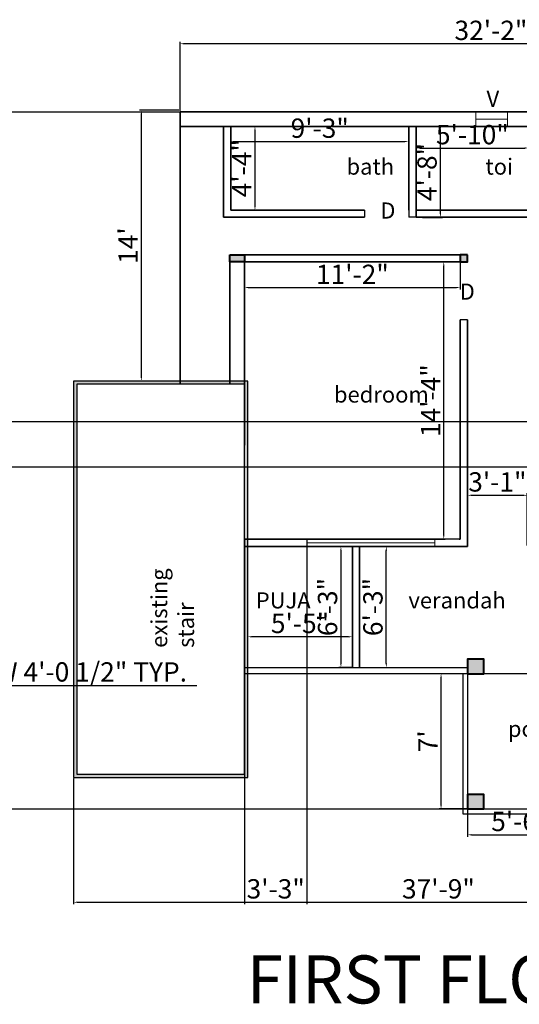
# Model space of a CAD drawing. Units: inches. Extents: x 1989 to 3287, y 1752 to 2384.
# Tile 4 of 5: x 2638 to 2948, y 1752 to 2364. Entities that reach past the tile are written whole.
import ezdxf

# ---------------------------------------------------------------- set-up
doc = ezdxf.new("R2010")
doc.units = ezdxf.units.IN
for name, color, linetype, lineweight in [('A-ANNO-DIMS', 2, 'Continuous', 18), ('A-ANNO-TEXT', 7, 'Continuous', 18), ('A-AREA-IDEN', 7, 'Continuous', 18), ('A-COLS', 1, 'Continuous', 40), ('A-COLS-PATT', 8, 'Continuous', 13), ('A-DOOR', 3, 'Continuous', 25), ('A-FLOR-EDGE', 7, 'Continuous', 25), ('A-FLOR-PATT', 252, 'Continuous', 13), ('A-FLOR-STRS', 7, 'Continuous', 25), ('A-GLAZ', 4, 'Continuous', 18), ('A-WALL', 7, 'Continuous', 35)]:
    doc.layers.add(name, color=color, linetype=linetype, lineweight=lineweight)
doc.styles.get("Standard").update_dxf_attribs({"font": 'arial.ttf'})
doc.dimstyles.new('ISO-25', dxfattribs={"dimtxt": 12, "dimasz": 2.5, "dimexe": 1.25, "dimexo": 0.625, "dimtad": 1, "dimdec": 0, "dimlunit": 4, "dimtxsty": 'Standard', "dimcen": 2.5, "dimadec": 0, "dimazin": 0, "dimtfac": 1, "dimtdec": 0, "dimtmove": 0, "dimatfit": 3, "dimfxl": 1, "dimarcsym": 0})

# ---------------------------------------------------------------- blocks, each defined once
blk = doc.blocks.new('*D18')
at = {"layer": 'A-ANNO-DIMS', "color": 0, "lineweight": -2, "transparency": 16777216}
for p, q in [((2915.08, 1957.68), (2898.02, 1957.68)), ((2899.27, 1876.18), (2899.27, 1955.18)), ((2915.08, 1873.68), (2898.02, 1873.68))]:
    blk.add_line(p, q, dxfattribs=at)
at = {"layer": 'A-ANNO-DIMS', "color": 0, "transparency": 16777216}
for points in [[(2898.85, 1955.18), (2899.68, 1955.18), (2899.27, 1957.68)], [(2898.85, 1876.18), (2899.68, 1876.18), (2899.27, 1873.68)]]:
    blk.add_solid(points, dxfattribs=at)
at = {"layer": 'Defpoints', "color": 0, "transparency": 16777216}
for p in [(2899.27, 1957.68), (2915.71, 1957.68), (2915.71, 1873.68)]:
    blk.add_point(p, dxfattribs=at)
at = {"layer": 'A-ANNO-DIMS', "color": 0, "transparency": 16777216, "insert": (2892.64, 1915.68), "char_height": 12, "attachment_point": 5, "rotation": 90}
blk.add_mtext("7'", dxfattribs=at)
blk = doc.blocks.new('*D19')
at = {"layer": 'A-ANNO-DIMS', "color": 0, "lineweight": -2, "transparency": 16777216}
for p, q in [((2915.71, 1873.05), (2915.71, 1856.37)), ((2981.21, 1873.05), (2981.21, 1856.37)), ((2918.21, 1857.62), (2978.71, 1857.62))]:
    blk.add_line(p, q, dxfattribs=at)
at = {"layer": 'A-ANNO-DIMS', "color": 0, "transparency": 16777216}
for points in [[(2918.21, 1858.04), (2918.21, 1857.2), (2915.71, 1857.62)], [(2978.71, 1858.04), (2978.71, 1857.2), (2981.21, 1857.62)]]:
    blk.add_solid(points, dxfattribs=at)
at = {"layer": 'Defpoints', "color": 0, "transparency": 16777216}
for p in [(2915.71, 1873.68), (2981.21, 1873.68), (2981.21, 1857.62)]:
    blk.add_point(p, dxfattribs=at)
at = {"layer": 'A-ANNO-DIMS', "color": 0, "transparency": 16777216, "insert": (2948.46, 1864.37), "char_height": 12, "attachment_point": 5}
blk.add_mtext('5\'-6"', dxfattribs=at)
blk = doc.blocks.new('*D24')
at = {"layer": 'A-ANNO-DIMS', "color": 0, "lineweight": -2, "transparency": 16777216}
for p, q in [((2910.58, 2213.45), (2899.68, 2213.45)), ((2900.93, 2043.68), (2900.93, 2210.95)), ((2910.58, 2041.18), (2899.68, 2041.18))]:
    blk.add_line(p, q, dxfattribs=at)
at = {"layer": 'A-ANNO-DIMS', "color": 0, "transparency": 16777216}
for points in [[(2900.52, 2210.95), (2901.35, 2210.95), (2900.93, 2213.45)], [(2900.52, 2043.68), (2901.35, 2043.68), (2900.93, 2041.18)]]:
    blk.add_solid(points, dxfattribs=at)
at = {"layer": 'Defpoints', "color": 0, "transparency": 16777216}
for p in [(2900.93, 2213.45), (2911.21, 2213.45), (2911.21, 2041.18)]:
    blk.add_point(p, dxfattribs=at)
at = {"layer": 'A-ANNO-DIMS', "color": 0, "transparency": 16777216, "insert": (2894.28, 2127.31), "char_height": 12, "attachment_point": 5, "rotation": 90}
blk.add_mtext('14\'-4"', dxfattribs=at)
blk = doc.blocks.new('*D25')
at = {"layer": 'A-ANNO-DIMS', "color": 0, "lineweight": -2, "transparency": 16777216}
for p, q in [((2777.21, 2212.82), (2777.21, 2196.3)), ((2911.21, 2212.82), (2911.21, 2196.3)), ((2779.71, 2197.55), (2908.71, 2197.55))]:
    blk.add_line(p, q, dxfattribs=at)
at = {"layer": 'A-ANNO-DIMS', "color": 0, "transparency": 16777216}
for points in [[(2779.71, 2197.97), (2779.71, 2197.13), (2777.21, 2197.55)], [(2908.71, 2197.97), (2908.71, 2197.13), (2911.21, 2197.55)]]:
    blk.add_solid(points, dxfattribs=at)
at = {"layer": 'Defpoints', "color": 0, "transparency": 16777216}
for p in [(2777.21, 2213.45), (2911.21, 2213.45), (2911.21, 2197.55)]:
    blk.add_point(p, dxfattribs=at)
at = {"layer": 'A-ANNO-DIMS', "color": 0, "transparency": 16777216, "insert": (2844.21, 2204.2), "char_height": 12, "attachment_point": 5}
blk.add_mtext('11\'-2"', dxfattribs=at)
blk = doc.blocks.new('*D26')
at = {"layer": 'A-ANNO-DIMS', "color": 0, "lineweight": -2, "transparency": 16777216}
for p, q in [((2736.58, 2307.68), (2711.96, 2307.68)), ((2713.21, 2141.99), (2713.21, 2305.18)), ((2736.58, 2139.49), (2711.96, 2139.49))]:
    blk.add_line(p, q, dxfattribs=at)
at = {"layer": 'A-ANNO-DIMS', "color": 0, "transparency": 16777216}
for points in [[(2712.79, 2305.18), (2713.63, 2305.18), (2713.21, 2307.68)], [(2712.79, 2141.99), (2713.63, 2141.99), (2713.21, 2139.49)]]:
    blk.add_solid(points, dxfattribs=at)
at = {"layer": 'Defpoints', "color": 0, "transparency": 16777216}
for p in [(2713.21, 2307.68), (2737.21, 2307.68), (2737.21, 2139.49)]:
    blk.add_point(p, dxfattribs=at)
at = {"layer": 'A-ANNO-DIMS', "color": 0, "transparency": 16777216, "insert": (2706.56, 2223.59), "char_height": 12, "attachment_point": 5, "rotation": 90}
blk.add_mtext("14'", dxfattribs=at)
blk = doc.blocks.new('*D27')
at = {"layer": 'A-ANNO-DIMS', "color": 0, "lineweight": -2, "transparency": 16777216}
for p, q in [((2737.21, 2307.3), (2737.21, 2350.26)), ((3120.71, 2349.01), (2739.71, 2349.01)), ((3123.21, 2307.3), (3123.21, 2350.26))]:
    blk.add_line(p, q, dxfattribs=at)
at = {"layer": 'A-ANNO-DIMS', "color": 0, "transparency": 16777216}
for points in [[(2739.71, 2349.43), (2739.71, 2348.6), (2737.21, 2349.01)], [(3120.71, 2349.43), (3120.71, 2348.6), (3123.21, 2349.01)]]:
    blk.add_solid(points, dxfattribs=at)
at = {"layer": 'Defpoints', "color": 0, "transparency": 16777216}
for p in [(2737.21, 2349.01), (2737.21, 2306.68), (3123.21, 2306.68)]:
    blk.add_point(p, dxfattribs=at)
at = {"layer": 'A-ANNO-DIMS', "color": 0, "transparency": 16777216, "insert": (2930.21, 2355.77), "char_height": 12, "attachment_point": 5}
blk.add_mtext('32\'-2"', dxfattribs=at)
blk = doc.blocks.new('*D30')
at = {"layer": 'A-ANNO-DIMS', "color": 0, "lineweight": -2, "transparency": 16777216}
for p, q in [((2887.74, 2297.53), (2900.1, 2297.53)), ((2898.85, 2243.64), (2898.85, 2295.03)), ((2887.74, 2241.14), (2900.1, 2241.14))]:
    blk.add_line(p, q, dxfattribs=at)
at = {"layer": 'A-ANNO-DIMS', "color": 0, "transparency": 16777216}
for points in [[(2898.44, 2295.03), (2899.27, 2295.03), (2898.85, 2297.53)], [(2898.44, 2243.64), (2899.27, 2243.64), (2898.85, 2241.14)]]:
    blk.add_solid(points, dxfattribs=at)
at = {"layer": 'Defpoints', "color": 0, "transparency": 16777216}
for p in [(2887.11, 2297.53), (2898.85, 2297.53), (2887.11, 2241.14)]:
    blk.add_point(p, dxfattribs=at)
at = {"layer": 'A-ANNO-DIMS', "color": 0, "transparency": 16777216, "insert": (2892.1, 2269.33), "char_height": 12, "attachment_point": 5, "rotation": 90}
blk.add_mtext('4\'-8"', dxfattribs=at)
blk = doc.blocks.new('*D39')
at = {"layer": 'A-ANNO-DIMS', "color": 0, "lineweight": -2, "transparency": 16777216}
for p, q in [((2883.71, 2297.05), (2883.71, 2282.99)), ((2953.71, 2297.05), (2953.71, 2282.99)), ((2886.21, 2284.24), (2951.21, 2284.24))]:
    blk.add_line(p, q, dxfattribs=at)
at = {"layer": 'A-ANNO-DIMS', "color": 0, "transparency": 16777216}
for points in [[(2886.21, 2284.65), (2886.21, 2283.82), (2883.71, 2284.24)], [(2951.21, 2284.65), (2951.21, 2283.82), (2953.71, 2284.24)]]:
    blk.add_solid(points, dxfattribs=at)
at = {"layer": 'Defpoints', "color": 0, "transparency": 16777216}
for p in [(2883.71, 2297.68), (2953.71, 2297.68), (2953.71, 2284.24)]:
    blk.add_point(p, dxfattribs=at)
at = {"layer": 'A-ANNO-DIMS', "color": 0, "transparency": 16777216, "insert": (2918.71, 2290.99), "char_height": 12, "attachment_point": 5}
blk.add_mtext('5\'-10"', dxfattribs=at)
blk = doc.blocks.new('*D40')
at = {"layer": 'A-ANNO-DIMS', "color": 0, "lineweight": -2, "transparency": 16777216}
for p, q in [((2768.71, 2297.05), (2768.71, 2287)), ((2879.21, 2297.05), (2879.21, 2287)), ((2771.21, 2288.25), (2876.71, 2288.25))]:
    blk.add_line(p, q, dxfattribs=at)
at = {"layer": 'A-ANNO-DIMS', "color": 0, "transparency": 16777216}
for points in [[(2771.21, 2288.66), (2771.21, 2287.83), (2768.71, 2288.25)], [(2876.71, 2288.66), (2876.71, 2287.83), (2879.21, 2288.25)]]:
    blk.add_solid(points, dxfattribs=at)
at = {"layer": 'Defpoints', "color": 0, "transparency": 16777216}
for p in [(2768.71, 2297.68), (2879.21, 2297.68), (2879.21, 2288.25)]:
    blk.add_point(p, dxfattribs=at)
at = {"layer": 'A-ANNO-DIMS', "color": 0, "transparency": 16777216, "insert": (2823.96, 2295), "char_height": 12, "attachment_point": 5}
blk.add_mtext('9\'-3"', dxfattribs=at)
blk = doc.blocks.new('*D41')
at = {"layer": 'A-ANNO-DIMS', "color": 0, "lineweight": -2, "transparency": 16777216}
for p, q in [((2769.33, 2297.68), (2784.99, 2297.68)), ((2783.74, 2295.18), (2783.74, 2248.18)), ((2769.33, 2245.68), (2784.99, 2245.68))]:
    blk.add_line(p, q, dxfattribs=at)
at = {"layer": 'A-ANNO-DIMS', "color": 0, "transparency": 16777216}
for points in [[(2783.33, 2295.18), (2784.16, 2295.18), (2783.74, 2297.68)], [(2783.33, 2248.18), (2784.16, 2248.18), (2783.74, 2245.68)]]:
    blk.add_solid(points, dxfattribs=at)
at = {"layer": 'Defpoints', "color": 0, "transparency": 16777216}
for p in [(2768.71, 2297.68), (2768.71, 2245.68), (2783.74, 2245.68)]:
    blk.add_point(p, dxfattribs=at)
at = {"layer": 'A-ANNO-DIMS', "color": 0, "transparency": 16777216, "insert": (2777.12, 2271.68), "char_height": 12, "attachment_point": 5, "rotation": 90}
blk.add_mtext('4\'-4"', dxfattribs=at)
blk = doc.blocks.new('*D44')
at = {"layer": 'A-ANNO-DIMS', "color": 0, "lineweight": -2, "transparency": 16777216}
for p, q in [((2779.21, 1962.17), (2779.21, 1981.88)), ((2844.21, 1962.17), (2844.21, 1981.88)), ((2841.71, 1980.63), (2781.71, 1980.63))]:
    blk.add_line(p, q, dxfattribs=at)
at = {"layer": 'A-ANNO-DIMS', "color": 0, "transparency": 16777216}
for points in [[(2781.71, 1981.05), (2781.71, 1980.22), (2779.21, 1980.63)], [(2841.71, 1981.05), (2841.71, 1980.22), (2844.21, 1980.63)]]:
    blk.add_solid(points, dxfattribs=at)
at = {"layer": 'Defpoints', "color": 0, "transparency": 16777216}
for p in [(2779.21, 1980.63), (2779.21, 1961.55), (2844.21, 1961.55)]:
    blk.add_point(p, dxfattribs=at)
at = {"layer": 'A-ANNO-DIMS', "color": 0, "transparency": 16777216, "insert": (2811.71, 1987.36), "char_height": 12, "attachment_point": 5}
blk.add_mtext('5\'-5"', dxfattribs=at)
blk = doc.blocks.new('*D45')
at = {"layer": 'A-ANNO-DIMS', "color": 0, "lineweight": -2, "transparency": 16777216}
for p, q in [((2843.58, 2036.68), (2835.86, 2036.68)), ((2837.11, 2034.18), (2837.11, 1964.05)), ((2843.58, 1961.55), (2835.86, 1961.55))]:
    blk.add_line(p, q, dxfattribs=at)
at = {"layer": 'A-ANNO-DIMS', "color": 0, "transparency": 16777216}
for points in [[(2836.69, 2034.18), (2837.52, 2034.18), (2837.11, 2036.68)], [(2836.69, 1964.05), (2837.52, 1964.05), (2837.11, 1961.55)]]:
    blk.add_solid(points, dxfattribs=at)
at = {"layer": 'Defpoints', "color": 0, "transparency": 16777216}
for p in [(2844.21, 2036.68), (2837.11, 1961.55), (2844.21, 1961.55)]:
    blk.add_point(p, dxfattribs=at)
at = {"layer": 'A-ANNO-DIMS', "color": 0, "transparency": 16777216, "insert": (2830.35, 1999.11), "char_height": 12, "attachment_point": 5, "rotation": 90}
blk.add_mtext('6\'-3"', dxfattribs=at)
blk = doc.blocks.new('*D46')
at = {"layer": 'A-ANNO-DIMS', "color": 0, "lineweight": -2, "transparency": 16777216}
for p, q in [((2849.33, 2036.68), (2866.53, 2036.68)), ((2865.28, 1964.05), (2865.28, 2034.18)), ((2849.33, 1961.55), (2866.53, 1961.55))]:
    blk.add_line(p, q, dxfattribs=at)
at = {"layer": 'A-ANNO-DIMS', "color": 0, "transparency": 16777216}
for points in [[(2864.86, 2034.18), (2865.69, 2034.18), (2865.28, 2036.68)], [(2864.86, 1964.05), (2865.69, 1964.05), (2865.28, 1961.55)]]:
    blk.add_solid(points, dxfattribs=at)
at = {"layer": 'Defpoints', "color": 0, "transparency": 16777216}
for p in [(2848.71, 2036.68), (2865.28, 2036.68), (2848.71, 1961.55)]:
    blk.add_point(p, dxfattribs=at)
at = {"layer": 'A-ANNO-DIMS', "color": 0, "transparency": 16777216, "insert": (2858.52, 1999.11), "char_height": 12, "attachment_point": 5, "rotation": 90}
blk.add_mtext('6\'-3"', dxfattribs=at)
blk = doc.blocks.new('*D47')
at = {"layer": 'A-ANNO-DIMS', "color": 0, "lineweight": -2, "transparency": 16777216}
for p, q in [((2915.71, 2037.3), (2915.71, 2069.77)), ((2918.21, 2068.52), (2950.21, 2068.52)), ((2952.71, 2037.3), (2952.71, 2069.77))]:
    blk.add_line(p, q, dxfattribs=at)
at = {"layer": 'A-ANNO-DIMS', "color": 0, "transparency": 16777216}
for points in [[(2918.21, 2068.93), (2918.21, 2068.1), (2915.71, 2068.52)], [(2950.21, 2068.93), (2950.21, 2068.1), (2952.71, 2068.52)]]:
    blk.add_solid(points, dxfattribs=at)
at = {"layer": 'Defpoints', "color": 0, "transparency": 16777216}
for p in [(2952.71, 2068.52), (2915.71, 2036.68), (2952.71, 2036.68)]:
    blk.add_point(p, dxfattribs=at)
at = {"layer": 'A-ANNO-DIMS', "color": 0, "transparency": 16777216, "insert": (2934.21, 2075.27), "char_height": 12, "attachment_point": 5}
blk.add_mtext('3\'-1"', dxfattribs=at)
blk = doc.blocks.new('VENT-TOILET')
blk.add_line((0, 4.5), (19.78, 4.5))
blk.add_lwpolyline([(0, 0), (19.78, 0), (19.78, 9), (0, 9)], close=True)
blk = doc.blocks.new('WIN-BEDROOM-VERANDAH')
for p, q in [((0, 0), (0, 4.5)), ((0, 2.25), (79.39, 2.25)), ((79.39, 0), (79.39, 4.5))]:
    blk.add_line(p, q)
blk = doc.blocks.new('COLUMN-10X9')
blk.add_lwpolyline([(0, 0), (10, 0), (10, 9), (0, 9)], close=True)
blk = doc.blocks.new('*D55')
at = {"layer": 'A-ANNO-DIMS', "color": 0, "lineweight": -2, "transparency": 16777216}
for p, q in [((2462.14, 1957.05), (2462.14, 1949.16)), ((2510.63, 1957.05), (2510.63, 1949.16)), ((2464.64, 1950.41), (2508.13, 1950.41)), ((2510.63, 1950.41), (2747.67, 1950.41))]:
    blk.add_line(p, q, dxfattribs=at)
at = {"layer": 'A-ANNO-DIMS', "color": 0, "transparency": 16777216}
for points in [[(2464.64, 1950.82), (2464.64, 1949.99), (2462.14, 1950.41)], [(2508.13, 1950.82), (2508.13, 1949.99), (2510.63, 1950.41)]]:
    blk.add_solid(points, dxfattribs=at)
at = {"layer": 'Defpoints', "color": 0, "transparency": 16777216}
for p in [(2462.14, 1957.68), (2510.63, 1957.68), (2510.63, 1950.41)]:
    blk.add_point(p, dxfattribs=at)
at = {"layer": 'A-ANNO-DIMS', "color": 0, "transparency": 16777216, "insert": (2630.4, 1957.24), "char_height": 12, "attachment_point": 5}
blk.add_mtext('STAIR WINDOW 4\'-0 1/2" TYP.', dxfattribs=at)
blk = doc.blocks.new('*D64')
at = {"layer": 'A-ANNO-DIMS', "color": 0, "lineweight": -2, "transparency": 16777216}
for p, q in [((2521.26, 2306.68), (3180.41, 2306.68)), ((3179.16, 1876.18), (3179.16, 2304.18)), ((2379.26, 1873.68), (3180.41, 1873.68))]:
    blk.add_line(p, q, dxfattribs=at)
at = {"layer": 'A-ANNO-DIMS', "color": 0, "transparency": 16777216}
for points in [[(3178.74, 2304.18), (3179.58, 2304.18), (3179.16, 2306.68)], [(3178.74, 1876.18), (3179.58, 1876.18), (3179.16, 1873.68)]]:
    blk.add_solid(points, dxfattribs=at)
at = {"layer": 'Defpoints', "color": 0, "transparency": 16777216}
for p in [(2520.64, 2306.68), (3179.16, 2306.68), (2378.64, 1873.68)]:
    blk.add_point(p, dxfattribs=at)
at = {"layer": 'A-ANNO-DIMS', "color": 0, "transparency": 16777216, "insert": (3172.4, 2090.18), "char_height": 12, "attachment_point": 5, "rotation": 90}
blk.add_mtext('36\'-1"', dxfattribs=at)
blk = doc.blocks.new('*D65')
at = {"layer": 'A-ANNO-DIMS', "color": 0, "lineweight": -2, "transparency": 16777216}
for p, q in [((3124.21, 2069.99), (3124.21, 1814.48)), ((2671.06, 1892.56), (2671.06, 1814.48)), ((2673.56, 1815.73), (3121.71, 1815.73))]:
    blk.add_line(p, q, dxfattribs=at)
at = {"layer": 'A-ANNO-DIMS', "color": 0, "transparency": 16777216}
for points in [[(2673.56, 1816.15), (2673.56, 1815.31), (2671.06, 1815.73)], [(3121.71, 1816.15), (3121.71, 1815.31), (3124.21, 1815.73)]]:
    blk.add_solid(points, dxfattribs=at)
at = {"layer": 'Defpoints', "color": 0, "transparency": 16777216}
for p in [(3124.21, 2070.62), (2671.06, 1893.19), (3124.21, 1815.73)]:
    blk.add_point(p, dxfattribs=at)
at = {"layer": 'A-ANNO-DIMS', "color": 0, "transparency": 16777216, "insert": (2897.63, 1822.49), "char_height": 12, "attachment_point": 5}
blk.add_mtext('37\'-9"', dxfattribs=at)
blk = doc.blocks.new('*D73')
at = {"layer": 'A-ANNO-DIMS', "color": 0, "lineweight": -2, "transparency": 16777216}
for p, q in [((2777.21, 2040.55), (2777.21, 1814.48)), ((2816.03, 2040.55), (2816.03, 1814.48)), ((2779.71, 1815.73), (2813.53, 1815.73))]:
    blk.add_line(p, q, dxfattribs=at)
at = {"layer": 'A-ANNO-DIMS', "color": 0, "transparency": 16777216}
for points in [[(2779.71, 1816.15), (2779.71, 1815.31), (2777.21, 1815.73)], [(2813.53, 1816.15), (2813.53, 1815.31), (2816.03, 1815.73)]]:
    blk.add_solid(points, dxfattribs=at)
at = {"layer": 'Defpoints', "color": 0, "transparency": 16777216}
for p in [(2777.21, 2041.18), (2816.03, 2041.18), (2816.03, 1815.73)]:
    blk.add_point(p, dxfattribs=at)
at = {"layer": 'A-ANNO-DIMS', "color": 0, "transparency": 16777216, "insert": (2796.62, 1822.49), "char_height": 12, "attachment_point": 5}
blk.add_mtext('3\'-3"', dxfattribs=at)
blk = doc.blocks.new('*D74')
at = {"layer": 'A-ANNO-DIMS', "color": 0, "lineweight": -2, "transparency": 16777216}
for p, q in [((3179.16, 2114.35), (3179.16, 2150.2)), ((2440.26, 2114.35), (3180.41, 2114.35)), ((3179.16, 2088.6), (3179.16, 2111.85)), ((2440.26, 2086.1), (3180.41, 2086.1))]:
    blk.add_line(p, q, dxfattribs=at)
at = {"layer": 'A-ANNO-DIMS', "color": 0, "transparency": 16777216}
for points in [[(3178.74, 2111.85), (3179.58, 2111.85), (3179.16, 2114.35)], [(3178.74, 2088.6), (3179.58, 2088.6), (3179.16, 2086.1)]]:
    blk.add_solid(points, dxfattribs=at)
at = {"layer": 'Defpoints', "color": 0, "transparency": 16777216}
for p in [(2439.64, 2114.35), (3179.16, 2114.35), (2439.64, 2086.1)]:
    blk.add_point(p, dxfattribs=at)
at = {"layer": 'A-ANNO-DIMS', "color": 0, "transparency": 16777216, "insert": (3172.51, 2133.53), "char_height": 12, "attachment_point": 5, "rotation": 90}
blk.add_mtext('2\'-4"', dxfattribs=at)

msp = doc.modelspace()

# ---------------------------------------------------------------- hatches: boundary and pattern name
at = {"layer": 'A-COLS-PATT'}
h = msp.add_hatch(dxfattribs=at)
h.set_pattern_fill('GRAVEL', color=256, scale=0.2)
h.paths.add_polyline_path([(2777.21, 2217.95), (2768.21, 2217.95), (2768.21, 2213.45), (2777.21, 2213.45)])
h.paths.add_polyline_path([(2915.71, 2217.95), (2911.21, 2217.95), (2911.21, 2213.45), (2915.71, 2213.45)])
h.paths.add_polyline_path([(2925.71, 1882.68), (2915.71, 1882.68), (2915.71, 1873.68), (2925.71, 1873.68)])
h.paths.add_polyline_path([(2981.21, 1882.68), (2971.21, 1882.68), (2971.21, 1873.68), (2981.21, 1873.68)])
h.paths.add_polyline_path([(2925.71, 1966.68), (2915.71, 1966.68), (2915.71, 1957.68), (2925.71, 1957.68)])
h.paths.add_polyline_path([(2981.21, 1966.68), (2971.21, 1966.68), (2971.21, 1957.68), (2981.21, 1957.68)])
h.paths.add_polyline_path([(3123.2, 1966.68), (3113.2, 1966.68), (3113.2, 1957.68), (3123.2, 1957.68)])
h.paths.add_polyline_path([(2962.71, 2041.18), (2957.21, 2041.18), (2957.21, 2045.68), (2952.71, 2045.68), (2952.71, 2036.68), (2962.71, 2036.68)])
h.paths.add_polyline_path([(3113.84, 2018.44), (3162.55, 2018.44), (3162.55, 2043.17), (3113.84, 2043.17)], flags=9)
at = {"layer": 'A-FLOR-PATT'}
h = msp.add_hatch(color=256, dxfattribs=at)
h.dxf.hatch_style = 1
h.paths.add_polyline_path([(2737.21, 2139.49), (2671.06, 2139.49), (2671.06, 1893.19), (2779.21, 1893.19), (2779.21, 2139.49), (2777.21, 2139.49), (2777.21, 2099.68), (2777.21, 1895.19), (2673.06, 1895.19), (2673.06, 2137.49), (2737.21, 2137.49)])
h.paths.add_polyline_path([(2768.21, 2139.49), (2737.21, 2139.49), (2737.21, 2137.49), (2768.21, 2137.49)], flags=17)
h.paths.add_polyline_path([(2777.21, 2139.49), (2768.21, 2139.49), (2768.21, 2137.49), (2777.21, 2137.49)], flags=17)

# ---------------------------------------------------------------- linework, layer by layer
at = {"layer": 'A-COLS'}
msp.add_line((2925.71, 1966.68), (2915.71, 1966.68), dxfattribs=at)
for points in [[(2768.21, 2217.95), (2777.21, 2217.95), (2777.21, 2213.45), (2768.21, 2213.45)], [(2915.71, 2217.95), (2911.21, 2217.95), (2911.21, 2213.45), (2915.71, 2213.45)], [(2915.71, 1873.68), (2925.71, 1873.68), (2925.71, 1882.68), (2915.71, 1882.68)]]:
    msp.add_lwpolyline(points, close=True, dxfattribs=at)
at = {"layer": 'A-DOOR'}
for p, q in [((2851.81, 2245.68), (2851.81, 2241.18)), ((2879.21, 2245.68), (2879.21, 2241.18)), ((2883.71, 2241.18), (2879.21, 2241.18))]:
    msp.add_line(p, q, dxfattribs=at)
for points in [[(2883.71, 2245.68), (2883.71, 2241.18), (2879.21, 2241.18)], [(2915.71, 2177.45), (2911.21, 2177.45)]]:
    msp.add_lwpolyline(points, dxfattribs=at)
at = {"layer": 'A-FLOR-EDGE'}
for p, q in [((2777.21, 1961.55), (2915.71, 1961.55)), ((2915.21, 1957.68), (2777.21, 1957.68)), ((2912.71, 1957.68), (2912.71, 1870.68)), ((3016.21, 1957.68), (2915.21, 1957.68)), ((2915.71, 1957.68), (2915.71, 1873.68)), ((2915.71, 1873.68), (2981.21, 1873.68)), ((2912.71, 1870.68), (2984.21, 1870.68))]:
    msp.add_line(p, q, dxfattribs=at)
at = {"layer": 'A-FLOR-STRS'}
for points in [[(2779.21, 2139.49), (2671.06, 2139.49), (2671.06, 1893.19), (2779.21, 1893.19)], [(2777.21, 2137.49), (2673.06, 2137.49), (2673.06, 1895.19), (2777.21, 1895.19)]]:
    msp.add_lwpolyline(points, close=True, dxfattribs=at)
at = {"layer": 'A-GLAZ'}
for points in [[(2911.21, 2136.11), (2911.21, 2167.31)], [(2915.71, 2167.31), (2915.71, 2136.11)]]:
    msp.add_lwpolyline(points, dxfattribs=at)
at = {"layer": 'A-WALL'}
for p, q in [((2746.21, 2297.68), (2737.21, 2297.68)), ((2764.21, 2297.68), (2764.21, 2241.18)), ((2816.71, 2297.68), (2768.71, 2297.68)), ((2768.71, 2297.68), (2768.71, 2245.68)), ((2909.21, 2297.68), (2879.21, 2297.68)), ((2879.21, 2297.68), (2879.21, 2245.68)), ((2883.71, 2297.68), (2883.71, 2241.18)), ((2953.71, 2297.68), (2913.71, 2297.68)), ((2768.71, 2245.68), (2784.71, 2245.68)), ((2883.71, 2245.68), (2909.21, 2245.68)), ((2909.21, 2245.68), (2913.71, 2245.68)), ((2913.71, 2245.68), (2958.21, 2245.68)), ((2764.21, 2241.18), (2784.71, 2241.18)), ((2883.71, 2241.18), (2953.71, 2241.18)), ((2768.21, 2137.49), (2768.21, 2217.95)), ((2915.71, 2217.95), (2768.21, 2217.95)), ((2915.71, 2217.95), (2915.71, 2213.45)), ((2777.21, 2099.68), (2777.21, 2213.45)), ((2911.21, 2213.45), (2777.21, 2213.45)), ((2911.21, 2177.45), (2911.21, 2099.68)), ((2915.71, 2177.45), (2915.71, 2099.68)), ((2911.21, 2090.68), (2911.21, 2099.68)), ((2911.21, 2090.68), (2911.21, 2041.18)), ((2901.87, 2041.18), (2777.21, 2041.18)), ((2910.58, 2041.18), (2911.21, 2041.18)), ((2905.21, 2036.68), (2777.21, 2036.68)), ((2777.21, 2036.68), (2844.21, 2036.68)), ((2844.21, 2036.68), (2844.21, 1961.55)), ((2848.71, 2036.68), (2848.71, 1961.55)), ((2905.21, 2036.68), (2915.71, 2036.68)), ((2844.21, 1971.68), (2844.21, 1961.55))]:
    msp.add_line(p, q, dxfattribs=at)
for points in [[(3123.21, 2090.68), (3123.21, 2306.68), (2737.21, 2306.68), (2737.21, 2137.49)], [(3114.21, 2099.68), (3114.21, 2297.68), (2746.21, 2297.68)], [(2768.71, 2245.68), (2851.81, 2245.68)], [(2851.81, 2241.18), (2768.71, 2241.18)], [(2915.71, 2099.68), (2915.71, 2036.68)]]:
    msp.add_lwpolyline(points, dxfattribs=at)

# ---------------------------------------------------------------- block references
at = {"layer": 'A-COLS'}
msp.add_blockref('COLUMN-10X9', (2915.71, 1957.68), dxfattribs=at)
at = {"layer": 'A-GLAZ'}
for name, p in [('VENT-TOILET', (2920.79, 2297.68)), ('WIN-BEDROOM-VERANDAH', (2816.03, 2036.68))]:
    msp.add_blockref(name, p, dxfattribs=at)

# ---------------------------------------------------------------- texts
at = {"layer": 'A-ANNO-TEXT', "attachment_point": 1}
for s, width, gutter_width, insert, char_height in [('V', 78.3523, 49.99, (2927.49, 2319.8), 10), ('D', 78.3523, 49.99, (2861.54, 2250.4), 10), ('D', 78.3523, 49.99, (2910.82, 2200.06), 10), ('FIRST FLOOR', 4273.6475, 149.09, (2778.54, 1782.67), 29.8187)]:
    msp.add_mtext_dynamic_manual_height_columns(s, width=width, gutter_width=gutter_width, heights=[0], dxfattribs=dict(at, insert=insert, char_height=char_height))
at = {"layer": 'A-ANNO-TEXT', "insert": (2719.25, 1973.76), "char_height": 9.9978, "attachment_point": 1, "rotation": 90}
msp.add_mtext_dynamic_manual_height_columns('existing stair', width=78.3523, gutter_width=49.99, heights=[0], dxfattribs=at)
at = {"layer": 'A-AREA-IDEN', "char_height": 9.998, "attachment_point": 1}
for s, insert in [('bath', (2840.57, 2277.69)), ('toi', (2926.82, 2277.69)), ('bedroom', (2832.76, 2136.11)), ('PUJA', (2784.24, 2008.24)), ('verandah', (2879.02, 2008.24)), ('porch', (2940.73, 1928.41))]:
    msp.add_mtext_dynamic_manual_height_columns(s, width=78.3523, gutter_width=49.99, heights=[0], dxfattribs=dict(at, insert=insert))

# ---------------------------------------------------------------- dimensions: what is measured, and where the dimension line sits
at = {"layer": 'A-ANNO-DIMS'}
for base, p1, p2, override, picture, middle in [((2737.21, 2349.01), (3123.21, 2306.68), (2737.21, 2306.68), {"dimclrd": 0, "dimclre": 0, "dimclrt": 0}, '*D27', (2930.21, 2355.77)), ((2879.20906953, 2288.24661815), (2768.70906953, 2297.67998165), (2879.20906953, 2297.67998165), {"dimclrd": 0, "dimclre": 0, "dimclrt": 0}, '*D40', (2823.95906953, 2295.00258677)), ((2953.71, 2284.24), (2883.71, 2297.68), (2953.71, 2297.68), {"dimclrd": 0, "dimclre": 0, "dimclrt": 0}, '*D39', (2918.71, 2290.99)), ((2911.21, 2197.55), (2777.21, 2213.45), (2911.21, 2213.45), {"dimclrd": 0, "dimclre": 0, "dimclrt": 0}, '*D25', (2844.21, 2204.2)), ((2952.71, 2068.52), (2915.71, 2036.68), (2952.71, 2036.68), {"dimclrd": 0, "dimclre": 0, "dimclrt": 0}, '*D47', (2934.21, 2075.27)), ((3124.2091, 1815.73), (2671.0578, 1893.1857), (3124.2091, 2070.6179), {"dimdec": 1, "dimlfac": 1, "dimrnd": 0, "dimzin": 1, "dimdsep": 46, "dimlunit": 4, "dimfrac": 2}, '*D65', (2897.6335, 1822.486)), ((2816.03, 1815.73), (2777.21, 2041.18), (2816.03, 2041.18), {"dimdec": 1, "dimlfac": 1, "dimrnd": 0, "dimzin": 1, "dimdsep": 46, "dimlunit": 4, "dimfrac": 2}, '*D73', (2796.62, 1822.49)), ((2779.21, 1980.63), (2844.21, 1961.55), (2779.21, 1961.55), {"dimclrd": 0, "dimclre": 0, "dimclrt": 0}, '*D44', (2811.71, 1987.36)), ((2981.20906953, 1857.62054686), (2915.70906953, 1873.67998165), (2981.20906953, 1873.67998165), {"dimclrd": 0, "dimclre": 0, "dimclrt": 0}, '*D19', (2948.45906953, 1864.37242271))]:
    dim = msp.add_linear_dim(base=base, p1=p1, p2=p2, dimstyle='ISO-25', override=override, dxfattribs=at)
    dim.commit()
    dim.dimension.update_dxf_attribs({"geometry": picture, "text_midpoint": middle})
for base, p1, p2, override, picture, middle in [((3179.16, 2306.68), (2378.64, 1873.68), (2520.64, 2306.68), {"dimdec": 1, "dimlfac": 1, "dimrnd": 0, "dimzin": 1, "dimdsep": 46, "dimlunit": 4, "dimfrac": 2}, '*D64', (3172.4, 2090.18)), ((2713.21, 2307.68), (2737.21, 2139.49), (2737.21, 2307.68), {"dimclrd": 0, "dimclre": 0, "dimclrt": 0}, '*D26', (2706.56, 2223.59)), ((2783.74, 2245.68), (2768.71, 2297.68), (2768.71, 2245.68), {"dimclrd": 0, "dimclre": 0, "dimclrt": 0}, '*D41', (2777.12, 2271.68)), ((2898.85, 2297.53), (2887.11, 2241.14), (2887.11, 2297.53), {"dimclrd": 0, "dimclre": 0, "dimclrt": 0}, '*D30', (2892.1, 2269.33)), ((2900.93, 2213.45), (2911.21, 2041.18), (2911.21, 2213.45), {"dimclrd": 0, "dimclre": 0, "dimclrt": 0}, '*D24', (2894.28, 2127.31)), ((3179.1591, 2114.3493), (2439.6365, 2086.1013), (2439.6365, 2114.3493), {"dimdec": 1, "dimlfac": 1, "dimrnd": 0, "dimzin": 1, "dimdsep": 46, "dimlunit": 4, "dimfrac": 2}, '*D74', (3172.5095, 2133.5261)), ((2837.11, 1961.55), (2844.21, 2036.68), (2844.21, 1961.55), {"dimclrd": 0, "dimclre": 0, "dimclrt": 0}, '*D45', (2830.35, 1999.11)), ((2865.28, 2036.68), (2848.71, 1961.55), (2848.71, 2036.68), {"dimclrd": 0, "dimclre": 0, "dimclrt": 0}, '*D46', (2858.52, 1999.11)), ((2899.27, 1957.68), (2915.71, 1873.68), (2915.71, 1957.68), {"dimclrd": 0, "dimclre": 0, "dimclrt": 0}, '*D18', (2892.64, 1915.68))]:
    dim = msp.add_linear_dim(base=base, p1=p1, p2=p2, angle=90, dimstyle='ISO-25', override=override, dxfattribs=at)
    dim.commit()
    dim.dimension.update_dxf_attribs({"geometry": picture, "text_midpoint": middle})
dim = msp.add_linear_dim(base=(2510.63, 1950.41), p1=(2462.14, 1957.68), p2=(2510.63, 1957.68), text='STAIR WINDOW <> TYP.', dimstyle='ISO-25', override={"dimdec": 1, "dimlfac": 1, "dimrnd": 0, "dimzin": 1, "dimdsep": 46, "dimlunit": 4, "dimfrac": 2}, dxfattribs=at)
dim.commit()
dim.dimension.update_dxf_attribs({"geometry": '*D55', "text_midpoint": (2630.4, 1957.24)})

doc.saveas('drawing.dxf')
